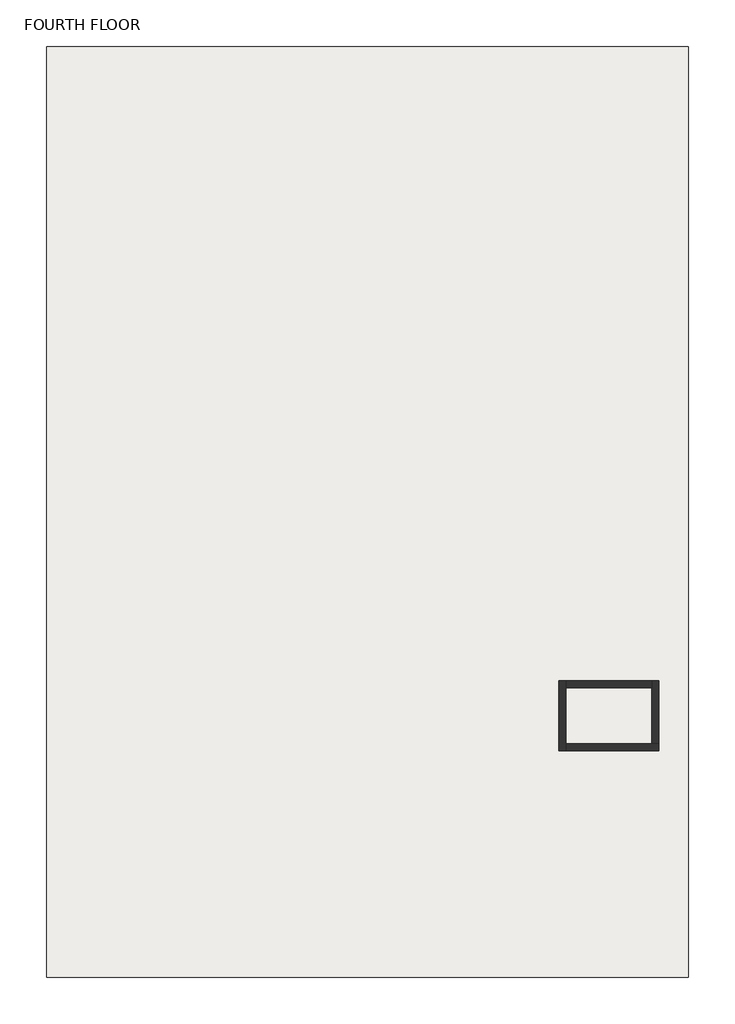
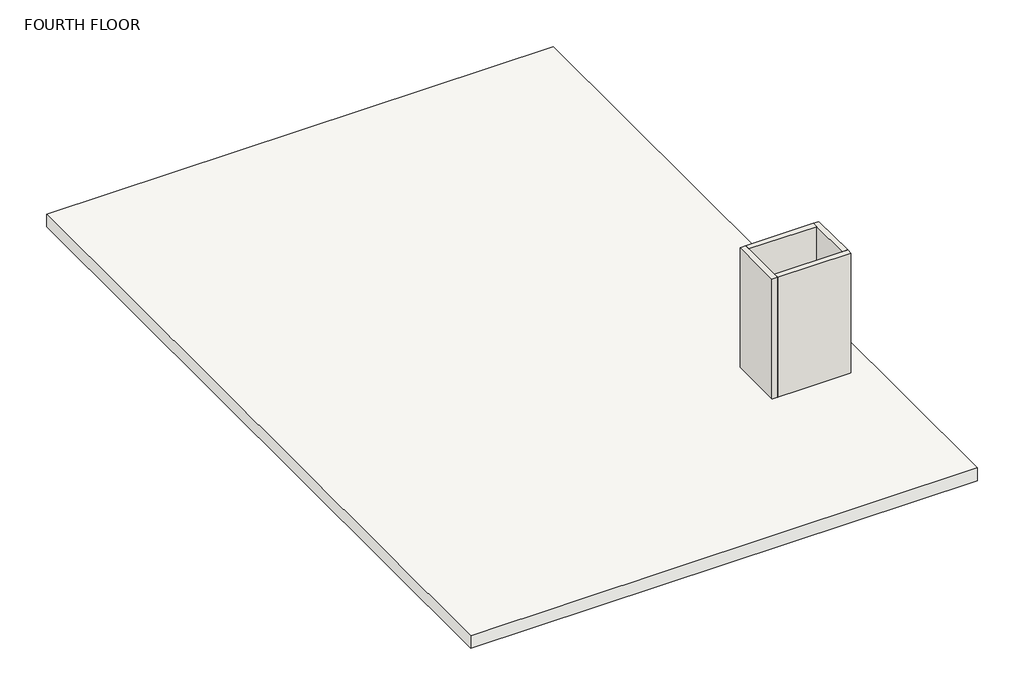
# One storey: 4 walls, 1 slab.
"""IFC4 building model written with IfcOpenShell, lengths in millimetres."""

from ifc_helpers import new_model, si_unit, frame, origin, place, context, project, spatial, polyline, outline, extrude, faceted_brep, element, save

model = new_model("IFC4")

# Units and contexts
model_context = context("Model", 3, world=origin())
ifc_project = project(units=[si_unit("LENGTHUNIT", "METRE", prefix="MILLI")], contexts=[model_context])

# Site, building, storey
site = spatial("IfcSite", under=ifc_project)
building = spatial("IfcBuilding", under=site)
storey = spatial("IfcBuildingStorey", under=building, Name="FOURTH FLOOR", Elevation=12801.6)

# Slab
placement = place(None, origin())
element("IfcSlab", 1, ObjectType="Generic - 12\"", at=placement, inside=storey, context=model_context, shape_type="SweptSolid", body=[
    extrude(outline(polyline([(4815.1311655, 8833.6177996), (4815.1311655, -7955.7822004), (-6765.9108866, -7955.7822004), (-6765.9108866, 8833.6177996), (4815.1311655, 8833.6177996)])), frame((0.0, 0.0, 12496.8), z_axis=(0.0, 0.0, 1.0), x_axis=(1.0, 0.0, 0.0)), (0.0, 0.0, 1.0), 304.8),
])

# Walls
element("IfcWall", 2, ObjectType="Generic - 5\"", at=placement, inside=storey, context=model_context, shape_type="Brep", body=[
    faceted_brep([(2479.6891134, -2605.6600272, 12801.6), (2479.6891134, -3866.3822004, 12801.6), (2479.6891134, -3866.3822004, 15697.2), (2479.6891134, -2605.6600272, 15697.2), (2606.6891134, -2605.6600272, 12801.6), (2606.6891134, -2605.6600272, 15697.2), (2606.6891134, -2732.6600272, 15697.2), (2606.6891134, -3739.3822004, 15697.2), (2606.6891134, -3866.3822004, 15697.2), (2606.6891134, -3866.3822004, 12801.6), (2606.6891134, -3739.3822004, 12801.6), (2606.6891134, -2732.6600272, 12801.6)], [[[0, 1, 2, 3]], [[4, 5, 6, 7, 8, 9, 10, 11]], [[1, 0, 4, 11, 10, 9]], [[3, 2, 8, 7, 6, 5]], [[2, 1, 9, 8]], [[0, 3, 5, 4]]]),
])
element("IfcWall", 3, ObjectType="Generic - 5\"", at=placement, inside=storey, context=model_context, shape_type="Brep", body=[
    faceted_brep([(2606.6891134, -3866.3822004, 12801.6), (4281.7311655, -3866.3822004, 12801.6), (4281.7311655, -3866.3822004, 15697.2), (2606.6891134, -3866.3822004, 15697.2), (2606.6891134, -3739.3822004, 12801.6), (2606.6891134, -3739.3822004, 15697.2), (4154.7311655, -3739.3822004, 15697.2), (4281.7311655, -3739.3822004, 15697.2), (4281.7311655, -3739.3822004, 12801.6), (4154.7311655, -3739.3822004, 12801.6)], [[[0, 1, 2, 3]], [[4, 5, 6, 7, 8, 9]], [[1, 0, 4, 9, 8]], [[3, 2, 7, 6, 5]], [[0, 3, 5, 4]], [[2, 1, 8, 7]]]),
])
element("IfcWall", 4, ObjectType="Generic - 5\"", at=placement, inside=storey, context=model_context, shape_type="Brep", body=[
    faceted_brep([(4281.7311655, -3739.3822004, 12801.6), (4281.7311655, -2605.6600272, 12801.6), (4281.7311655, -2605.6600272, 15697.2), (4281.7311655, -3739.3822004, 15697.2), (4154.7311655, -3739.3822004, 12801.6), (4154.7311655, -3739.3822004, 15697.2), (4154.7311655, -2732.6600272, 15697.2), (4154.7311655, -2605.6600272, 15697.2), (4154.7311655, -2605.6600272, 12801.6), (4154.7311655, -2732.6600272, 12801.6)], [[[0, 1, 2, 3]], [[4, 5, 6, 7, 8, 9]], [[1, 0, 4, 9, 8]], [[3, 2, 7, 6, 5]], [[0, 3, 5, 4]], [[2, 1, 8, 7]]]),
])
element("IfcWall", 5, ObjectType="Generic - 5\"", at=placement, inside=storey, context=model_context, shape_type="SweptSolid", body=[
    extrude(outline(polyline([(4154.7311655, -2732.6600272), (2606.6891134, -2732.6600272), (2606.6891134, -2605.6600272), (4154.7311655, -2605.6600272), (4154.7311655, -2732.6600272)])), frame((0.0, 0.0, 12801.6), z_axis=(0.0, 0.0, 1.0), x_axis=(1.0, 0.0, 0.0)), (0.0, 0.0, 1.0), 2895.6),
])

save(model, "model.ifc")

# Revit data of these elements
# Type "Generic - 12\""
#   Assembly Code = "B1010"
#   Function = 0
#   Layers, outside or top first: 1' - 0" no material (function 1)
# Type "Generic - 5\""
#   Assembly Code = "B2010"
#   Layers, outside or top first: 0' - 5" no material (function 1)
# Element 1 (IfcSlab, "Generic - 12\"")
#   Height Offset From Level = 0' - 0"
#   Phase Created = New Construction
#   Materials on its faces: "Default Floor"
# Elements 2, 3, 4, 5 (IfcWall, "Generic - 5\"")
#   Top Offset = -0' - 6"
#   Base Offset = 0' - 0"
#   wall height = 9' - 6"
#   Phase Created = New Construction
#   Base Constraint = FOURTH FLOOR
#   Top Constraint = ROOF
#   Materials on its faces: "Default Wall"
# Materials
#   "Default Floor": colour RGB 128 128 128, transparency 0, Cost = 0
#   "Default Wall": colour RGB 128 128 128, transparency 0, Cost = 0
